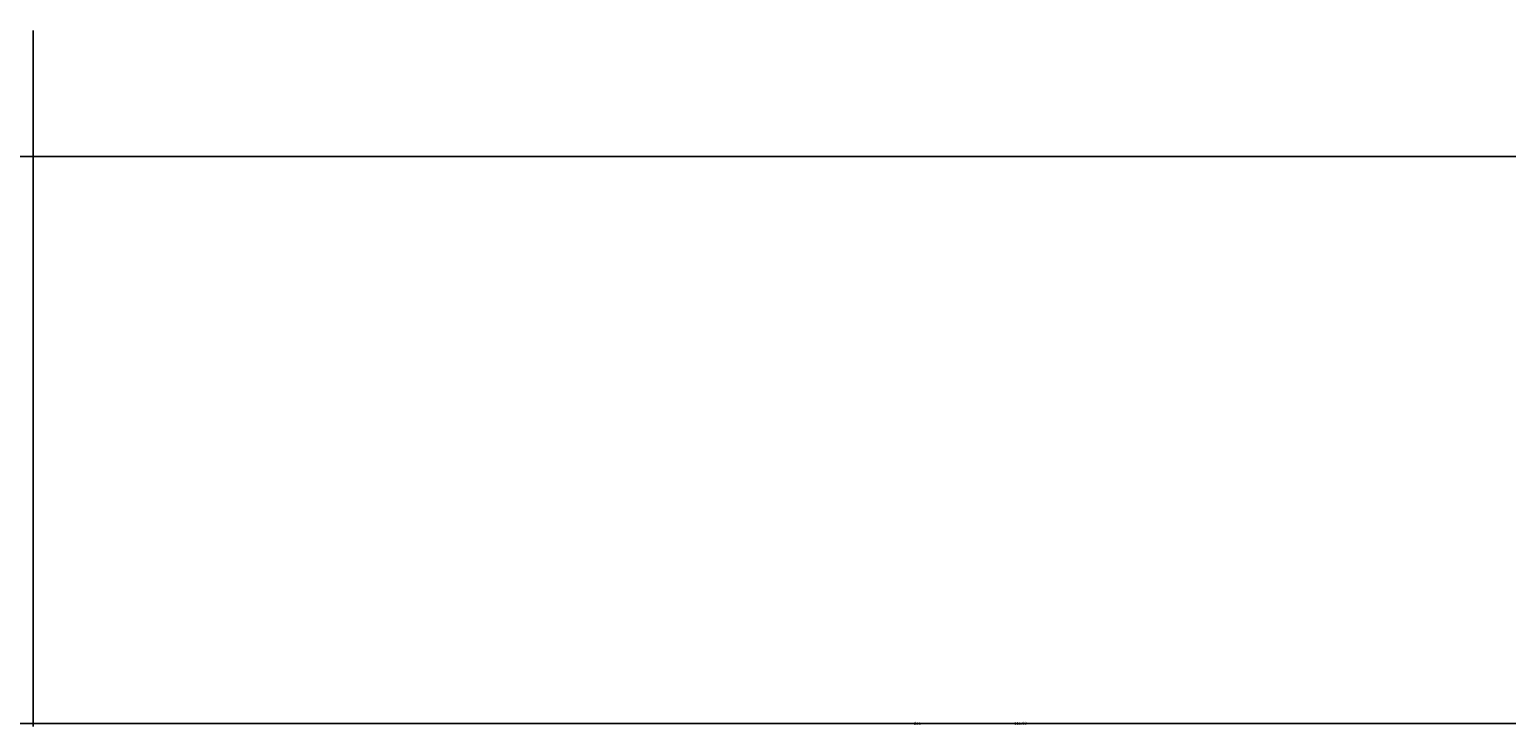
# Model space of a CAD drawing. Units: inches. Extents: x 4159 to 4826, y 299 to 1026.
# Tile 2 of 37: x 4268 to 4354, y 299 to 340. Entities that reach past the tile are written whole.
import ezdxf

# ---------------------------------------------------------------- set-up
doc = ezdxf.new("R2010")
doc.units = ezdxf.units.IN
doc.layers.add('A-ANNO-DIMS', color=2, linetype='Continuous', lineweight=18)
doc.styles.get("Standard").update_dxf_attribs({"font": 'arial.ttf'})
doc.dimstyles.get("Standard").update_dxf_attribs({"dimtxt": 0.18, "dimasz": 0.18, "dimexe": 0.18, "dimexo": 0.0625, "dimgap": 0.09, "dimtad": 0, "dimtih": 1, "dimtoh": 1, "dimdec": 4, "dimzin": 0, "dimdsep": 46, "dimtxsty": 'Standard', "dimcen": 0.09, "dimadec": 0, "dimazin": 0, "dimtfac": 1, "dimtdec": 4, "dimtofl": 0, "dimtmove": 0, "dimatfit": 3, "dimfxl": 1, "dimtolj": 1, "dimtzin": 0, "dimarcsym": 0})

# ---------------------------------------------------------------- blocks, each defined once
blk = doc.blocks.new('*D44')
at = {"layer": 'A-ANNO-DIMS', "color": 0, "lineweight": -2, "transparency": 16777216}
for p, q in [((4287.263, 963.093), (4158.88, 963.093)), ((4159.06, 962.913), (4159.06, 647.826)), ((4159.06, 332.375), (4159.06, 647.462)), ((4447.248, 332.195), (4158.88, 332.195))]:
    blk.add_line(p, q, dxfattribs=at)
at = {"layer": 'A-ANNO-DIMS', "color": 0, "transparency": 16777216}
for points in [[(4159.03, 962.913), (4159.09, 962.913), (4159.06, 963.093)], [(4159.03, 332.375), (4159.09, 332.375), (4159.06, 332.195)]]:
    blk.add_solid(points, dxfattribs=at)
at = {"layer": 'Defpoints', "color": 0, "transparency": 16777216}
for p in [(4287.326, 963.093), (4159.06, 332.195), (4447.31, 332.195)]:
    blk.add_point(p, dxfattribs=at)
at = {"layer": 'A-ANNO-DIMS', "color": 0, "transparency": 16777216, "insert": (4159.06, 647.644), "char_height": 0.18, "attachment_point": 5}
blk.add_mtext('\\A1;630.9', dxfattribs=at)
blk = doc.blocks.new('*D46')
at = {"layer": 'A-ANNO-DIMS', "color": 0, "lineweight": -2, "transparency": 16777216}
for p, q in [((4192.31, 392.192), (4192.31, 298.765)), ((4447.31, 332.133), (4447.31, 298.765)), ((4192.49, 298.945), (4319.519, 298.945)), ((4447.13, 298.945), (4320.101, 298.945))]:
    blk.add_line(p, q, dxfattribs=at)
at = {"layer": 'A-ANNO-DIMS', "color": 0, "transparency": 16777216}
for points in [[(4192.49, 298.975), (4192.49, 298.915), (4192.31, 298.945)], [(4447.13, 298.975), (4447.13, 298.915), (4447.31, 298.945)]]:
    blk.add_solid(points, dxfattribs=at)
at = {"layer": 'Defpoints', "color": 0, "transparency": 16777216}
for p in [(4192.31, 392.254), (4447.31, 332.195), (4447.31, 298.945)]:
    blk.add_point(p, dxfattribs=at)
at = {"layer": 'A-ANNO-DIMS', "color": 0, "transparency": 16777216, "insert": (4319.81, 298.945), "char_height": 0.18, "attachment_point": 5}
blk.add_mtext('\\A1;255', dxfattribs=at)
blk = doc.blocks.new('*D52')
at = {"layer": 'A-ANNO-DIMS', "color": 0, "lineweight": -2, "transparency": 16777216}
for p, q in [((4192.31, 392.192), (4192.31, 298.765)), ((4267.89, 339.581), (4267.89, 298.765)), ((4192.49, 298.945), (4229.707, 298.945)), ((4267.71, 298.945), (4230.493, 298.945))]:
    blk.add_line(p, q, dxfattribs=at)
at = {"layer": 'A-ANNO-DIMS', "color": 0, "transparency": 16777216}
for points in [[(4192.49, 298.975), (4192.49, 298.915), (4192.31, 298.945)], [(4267.71, 298.975), (4267.71, 298.915), (4267.89, 298.945)]]:
    blk.add_solid(points, dxfattribs=at)
at = {"layer": 'Defpoints', "color": 0, "transparency": 16777216}
for p in [(4192.31, 392.254), (4267.89, 339.644), (4267.89, 298.945)]:
    blk.add_point(p, dxfattribs=at)
at = {"layer": 'A-ANNO-DIMS', "color": 0, "transparency": 16777216, "insert": (4230.1, 298.945), "char_height": 0.18, "attachment_point": 5}
blk.add_mtext('\\A1;75.58', dxfattribs=at)
blk = doc.blocks.new('*D53')
at = {"layer": 'A-ANNO-DIMS', "color": 0, "lineweight": -2, "transparency": 16777216}
for p, q in [((4267.89, 339.581), (4267.89, 298.765)), ((4383.821, 339.581), (4383.821, 298.765)), ((4268.07, 298.945), (4325.4, 298.945)), ((4383.641, 298.945), (4326.311, 298.945))]:
    blk.add_line(p, q, dxfattribs=at)
at = {"layer": 'A-ANNO-DIMS', "color": 0, "transparency": 16777216}
for points in [[(4268.07, 298.975), (4268.07, 298.915), (4267.89, 298.945)], [(4383.641, 298.975), (4383.641, 298.915), (4383.821, 298.945)]]:
    blk.add_solid(points, dxfattribs=at)
at = {"layer": 'Defpoints', "color": 0, "transparency": 16777216}
for p in [(4267.89, 339.644), (4383.821, 339.644), (4383.821, 298.945)]:
    blk.add_point(p, dxfattribs=at)
at = {"layer": 'A-ANNO-DIMS', "color": 0, "transparency": 16777216, "insert": (4325.855, 298.945), "char_height": 0.18, "attachment_point": 5}
blk.add_mtext('\\A1;115.93', dxfattribs=at)

msp = doc.modelspace()

# ---------------------------------------------------------------- dimensions: what is measured, and where the dimension line sits
at = {"layer": 'A-ANNO-DIMS'}
dim = msp.add_linear_dim(base=(4159.06, 332.195), p1=(4287.326, 963.093), p2=(4447.31, 332.195), angle=90, dimstyle='Standard', override={"dimdec": 1, "dimlfac": 1, "dimrnd": 0, "dimzin": 0, "dimdsep": 46, "dimlunit": 2}, dxfattribs=at)
dim.commit()
dim.dimension.update_dxf_attribs({"geometry": '*D44', "text_midpoint": (4159.06, 647.644)})
for base, p1, p2, override, picture, middle in [((4447.31, 298.945), (4192.31, 392.254), (4447.31, 332.195), {"dimdec": 0, "dimlfac": 1, "dimrnd": 0, "dimzin": 0, "dimdsep": 46, "dimlunit": 2}, '*D46', (4319.81, 298.945)), ((4267.89, 298.945), (4192.31, 392.254), (4267.89, 339.644), {"dimdec": 2, "dimlfac": 1, "dimrnd": 0, "dimzin": 0, "dimdsep": 46, "dimlunit": 2}, '*D52', (4230.1, 298.945)), ((4383.821, 298.945), (4267.89, 339.644), (4383.821, 339.644), {"dimdec": 2, "dimlfac": 1, "dimrnd": 0, "dimzin": 0, "dimdsep": 46, "dimlunit": 2}, '*D53', (4325.855, 298.945))]:
    dim = msp.add_linear_dim(base=base, p1=p1, p2=p2, dimstyle='Standard', override=override, dxfattribs=at)
    dim.commit()
    dim.dimension.update_dxf_attribs({"geometry": picture, "text_midpoint": middle})

doc.saveas('drawing.dxf')
